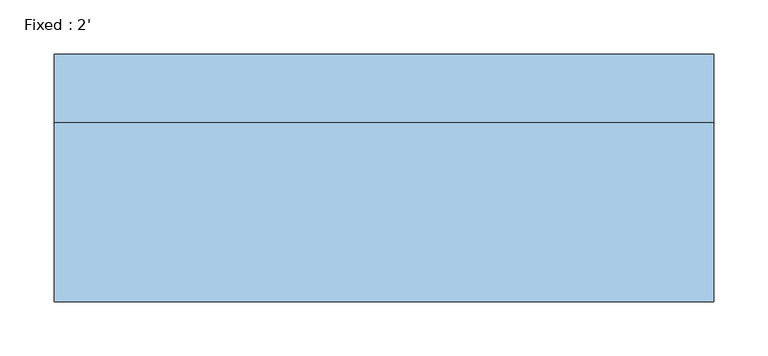
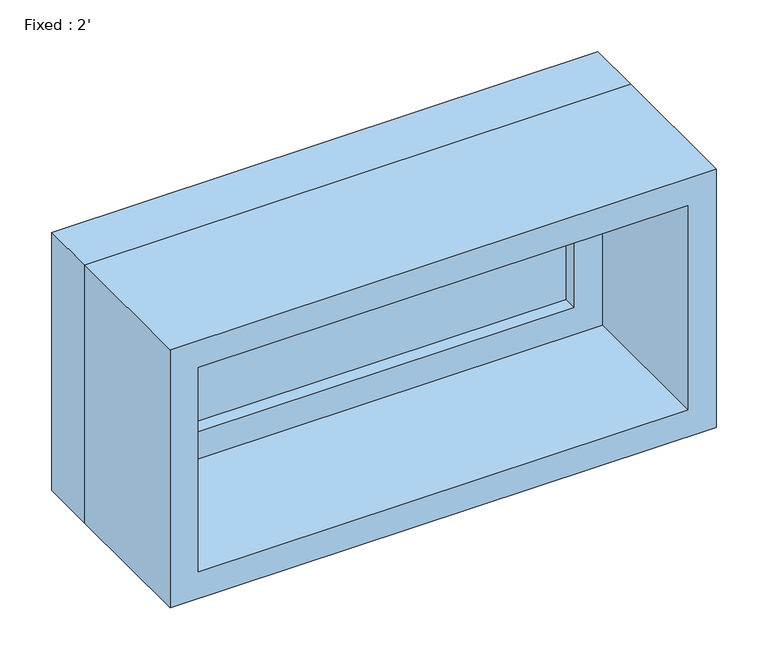
"""IFC4 building model written with IfcOpenShell, lengths in millimetres: window geometry, Fixed : 2'."""

from ifc_helpers import new_model, si_unit, frame, origin, place, context, project, spatial, polyline, outline, extrude, source, transform, mapped, element, save


def fixed_2_8c8825d0(model_context):
    return source(origin(), model_context, "Body", "SweptSolid", [
        extrude(outline(polyline([(203.2, 66.675), (-279.4, 66.675), (-279.4, 79.375), (203.2, 79.375), (203.2, 66.675)])), frame((0.0, 0.0, 977.9), z_axis=(0.0, 0.0, 1.0), x_axis=(1.0, 0.0, 0.0)), (0.0, 0.0, 1.0), 177.8),
        extrude(outline(polyline([(1200.15, -323.85), (933.45, -323.85), (933.45, 247.65), (1200.15, 247.65), (1200.15, -323.85)]), holes=[polyline([(1155.7, -279.4), (1155.7, 203.2), (977.9, 203.2), (977.9, -279.4), (1155.7, -279.4)])]), frame((0.0, 50.8, 0.0), z_axis=(0.0, 1.0, 0.0), x_axis=(0.0, 0.0, 1.0)), (0.0, 0.0, 1.0), 44.45),
        extrude(outline(polyline([(1219.2, -342.9), (914.4, -342.9), (914.4, 266.7), (1219.2, 266.7), (1219.2, -342.9)]), holes=[polyline([(1187.45, -311.15), (1187.45, 234.95), (946.15, 234.95), (946.15, -311.15), (1187.45, -311.15)])]), frame((0.0, -114.3, 0.0), z_axis=(0.0, 1.0, 0.0), x_axis=(0.0, 0.0, 1.0)), (0.0, 0.0, 1.0), 165.1),
        extrude(outline(polyline([(1219.2, 266.7), (1219.2, -342.9), (914.4, -342.9), (914.4, 266.7), (1219.2, 266.7)]), holes=[polyline([(1200.15, 247.65), (933.45, 247.65), (933.45, -323.85), (1200.15, -323.85), (1200.15, 247.65)])]), frame((0.0, 50.8, 0.0), z_axis=(0.0, 1.0, 0.0), x_axis=(0.0, 0.0, 1.0)), (0.0, 0.0, 1.0), 63.5),
    ])


if __name__ == "__main__":
    model = new_model("IFC4")
    model_context = context("Model", 3, world=origin())
    ifc_project = project(units=[si_unit("LENGTHUNIT", "METRE", prefix="MILLI")], contexts=[model_context])
    site = spatial("IfcSite", under=ifc_project)
    building = spatial("IfcBuilding", under=site)
    placement = place(None, origin())
    fixed_2_shape = fixed_2_8c8825d0(model_context)
    element("IfcWindow", 1, ObjectType="Fixed : 2'", at=placement, inside=building, context=model_context, shape_type="MappedRepresentation", body=[
        mapped(fixed_2_shape, transform((0.0, 0.0, 0.0), x_axis=(1.0, 0.0, 0.0), y_axis=(0.0, 1.0, 0.0), z_axis=(0.0, 0.0, 1.0))),
    ])
    save(model, "model.ifc")

# Revit data of these elements
# Type "Fixed : 2'"
#   Type Mark = "21"
#   Construction Type Id = "GSP4R"
#   Assembly Code = "B2020100"
#   Analytic Construction = "1/8 in Pilkington single glazing"
#   Rough Height = 1' - 0"
#   Visual Light Transmittance = 0.9
#   Solar Heat Gain Coefficient = 0.78
#   Heat Transfer Coefficient (U) = 0.6496 BTU/(h·ft²·°F)
#   Height = 1' - 0"
#   Default Sill Height = 3' - 0"
#   Width = 2' - 0"
#   Window Inset = 0' - 0 3/4"
#   Define Thermal Properties by = 1
#   Glass Pane Material = Glass
#   Sash Material = Sash
#   Wall Closure = (empty or 0)
# Element 1 (IfcWindow, "Fixed : 2'")
#   Materials on its faces: "Sash", "Glass"
# Materials
#   "Glass": class "Glass", colour RGB 0 128 192, transparency 0.75, Description = "Soda Lime Glass", Cost = 0
#   "Sash": class "Wood", colour RGB 224 178 126, transparency 0, Cost = 0
